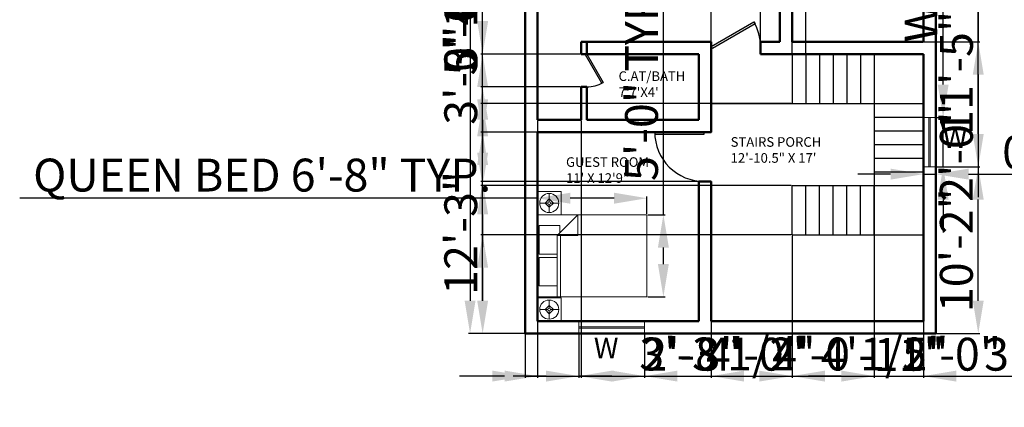
# Model space of a CAD drawing. Units: inches. Extents: x 1383 to 2465, y 1661 to 2415.
# Tile 1 of 4: x 1383 to 2102, y 1661 to 1944. Entities that reach past the tile are written whole.
import ezdxf

# ---------------------------------------------------------------- set-up
doc = ezdxf.new("R2010")
doc.units = ezdxf.units.IN
for name, color, linetype, lineweight in [('A-ANNO-DIMS', 2, 'Continuous', 18), ('A-ANNO-TEXT', 3, 'Continuous', 18), ('A-AREA-IDEN', 7, 'Continuous', 25), ('A-DOOR', 3, 'Continuous', 25), ('A-FLOR-STRS', 7, 'Continuous', 25), ('A-FURN', 8, 'Continuous', 18), ('A-GLAZ', 4, 'Continuous', 18), ('A-WALL', 7, 'Continuous', 50)]:
    doc.layers.add(name, color=color, linetype=linetype, lineweight=lineweight)
doc.styles.get("Standard").update_dxf_attribs({"font": 'arial.ttf'})
doc.dimstyles.new('ISO-25', dxfattribs={"dimtxt": 24, "dimasz": 24, "dimexe": 1.25, "dimexo": 0.625, "dimtad": 1, "dimdec": 0, "dimlunit": 3, "dimtxsty": 'Standard', "dimcen": 2.5, "dimadec": 0, "dimazin": 0, "dimtfac": 1, "dimtdec": 0, "dimtmove": 0, "dimatfit": 3, "dimfxl": 1, "dimarcsym": 0})

# ---------------------------------------------------------------- blocks, each defined once
blk = doc.blocks.new('*U7')
for p, q in [((0, 0), (0, -6)), ((40, 0), (40, -6))]:
    blk.add_line(p, q)
blk.add_lwpolyline([(0, 0), (34.64, 20), (35.52, 18.48), (0.87, -1.52)], close=True)
blk.add_arc((0, 0), 40, 0, 30)
blk = doc.blocks.new('*U6')
for p, q in [((0, 0), (0, 6)), ((40, 0), (40, 6))]:
    blk.add_line(p, q)
blk.add_lwpolyline([(0, 0), (0, -40), (1.75, -40), (1.75, 0)], close=True)
blk.add_arc((0, 0), 40, 270, 0)
blk = doc.blocks.new('*U3')
for p, q in [((0, 0), (0, -6)), ((40, 0), (40, -6))]:
    blk.add_line(p, q)
blk.add_lwpolyline([(0, 0), (34.6, 20), (35.5, 18.5), (0.9, -1.5)], close=True)
blk.add_arc((0, 0), 40, 0, 30)
blk = doc.blocks.new('Bed - Queen')
for p, q in [((0, -80.00003), (0, 0)), ((0, 0), (59.99999, 0)), ((59.99999, 0), (59.99999, -80.00003)), ((7.99999, -1.2), (28.79998, -1.2)), ((7.99999, -14.4), (7.99999, -1.2)), ((28.79998, -1.2), (28.79998, -14.4)), ((31.19999, -1.2), (51.99999, -1.2)), ((31.19999, -14.4), (31.19999, -1.2)), ((51.99999, -1.2), (51.99999, -16.4)), ((0, -14.4), (44.8, -14.4)), ((44.8, -16.8), (0, -16.8)), ((59.99999, -29.6), (44.8, -14.4)), ((44.8, -14.4), (44.8, -29.6)), ((51.99999, -16.4), (46.79936, -16.4)), ((44.8, -29.6), (59.99999, -29.6)), ((59.99999, -80.00003), (0, -80.00003))]:
    blk.add_line(p, q)
blk = doc.blocks.new('*D13')
at = {"layer": 'A-ANNO-DIMS', "color": 0, "lineweight": -2, "transparency": 16777216}
for p, q in [((1751.57, 2255.16), (1710.71, 2255.16)), ((1711.96, 2231.16), (1711.96, 1739.16)), ((1751.57, 1715.16), (1710.71, 1715.16))]:
    blk.add_line(p, q, dxfattribs=at)
at = {"layer": 'A-ANNO-DIMS', "color": 0, "transparency": 16777216}
for points in [[(1707.96, 2231.16), (1715.96, 2231.16), (1711.96, 2255.16)], [(1707.96, 1739.16), (1715.96, 1739.16), (1711.96, 1715.16)]]:
    blk.add_solid(points, dxfattribs=at)
at = {"layer": 'Defpoints', "color": 0, "transparency": 16777216}
for p in [(1752.19, 2255.16), (1711.96, 1715.16), (1752.19, 1715.16)]:
    blk.add_point(p, dxfattribs=at)
at = {"layer": 'A-ANNO-DIMS', "color": 0, "transparency": 16777216, "insert": (1699.13, 1985.16), "char_height": 24, "attachment_point": 5, "rotation": 90}
blk.add_mtext("45'", dxfattribs=at)
blk = doc.blocks.new('WIN-36IN')
for p, q in [((0, 36), (9, 36)), ((0, 0), (0, 36)), ((4, 0), (4, 36)), ((5, 36), (5, 0)), ((9, 36), (9, 0)), ((9, 0), (0, 0))]:
    blk.add_line(p, q)
blk = doc.blocks.new('Lamp - Table')
for p, q in [((-1, 0), (-7, 0)), ((0, 3), (-3, 0)), ((-3, 0), (0, -3)), ((0, 7), (0, 1)), ((3, 0), (0, 3)), ((0, -3), (3, 0)), ((1, 0), (7, 0)), ((0, -1), (0, -7))]:
    blk.add_line(p, q)
for radius in [7, 1]:
    blk.add_circle((0, 0), radius)
blk = doc.blocks.new('NIGHTSTAND-WITH-LAMP')
blk.add_lwpolyline([(0, 0), (17.23, 0), (17.23, 16.98), (0, 16.98)], close=True)
blk.add_blockref('Lamp - Table', (8.62, 8.49))
blk = doc.blocks.new('*D18')
at = {"layer": 'A-ANNO-DIMS', "color": 0, "lineweight": -2, "transparency": 16777216}
for p, q in [((2057.59, 1896.91), (2057.59, 2225.86)), ((2052.82, 1872.91), (2058.84, 1872.91)), ((2057.59, 1836.91), (2057.59, 1872.91)), ((2052.82, 1836.91), (2058.84, 1836.91)), ((2057.59, 1812.91), (2057.59, 1788.91))]:
    blk.add_line(p, q, dxfattribs=at)
at = {"layer": 'A-ANNO-DIMS', "color": 0, "transparency": 16777216}
for points in [[(2053.59, 1896.91), (2061.59, 1896.91), (2057.59, 1872.91)], [(2053.59, 1812.91), (2061.59, 1812.91), (2057.59, 1836.91)]]:
    blk.add_solid(points, dxfattribs=at)
at = {"layer": 'Defpoints', "color": 0, "transparency": 16777216}
for p in [(2052.19, 1872.91), (2057.59, 1872.91), (2052.19, 1836.91)]:
    blk.add_point(p, dxfattribs=at)
at = {"layer": 'A-ANNO-DIMS', "color": 0, "transparency": 16777216, "insert": (2044.54, 2073.39), "char_height": 24, "attachment_point": 5, "rotation": 90}
blk.add_mtext('WINDOW 3\'-0" TYP.', dxfattribs=at)
blk = doc.blocks.new('*D19')
at = {"layer": 'A-ANNO-DIMS', "color": 0, "lineweight": -2, "transparency": 16777216}
for p, q in [((2043.19, 1836.29), (2043.19, 1830.26)), ((2052.19, 1836.29), (2052.19, 1830.26)), ((2019.19, 1831.51), (1995.19, 1831.51)), ((2043.19, 1831.51), (2052.19, 1831.51)), ((2076.19, 1831.51), (2247.74, 1831.51))]:
    blk.add_line(p, q, dxfattribs=at)
at = {"layer": 'A-ANNO-DIMS', "color": 0, "transparency": 16777216}
for points in [[(2019.19, 1835.51), (2019.19, 1827.51), (2043.19, 1831.51)], [(2076.19, 1835.51), (2076.19, 1827.51), (2052.19, 1831.51)]]:
    blk.add_solid(points, dxfattribs=at)
at = {"layer": 'Defpoints', "color": 0, "transparency": 16777216}
for p in [(2043.19, 1836.91), (2052.19, 1836.91), (2052.19, 1831.51)]:
    blk.add_point(p, dxfattribs=at)
at = {"layer": 'A-ANNO-DIMS', "color": 0, "transparency": 16777216, "insert": (2173.96, 1844.39), "char_height": 24, "attachment_point": 5}
blk.add_mtext('0\'-9" TYP.', dxfattribs=at)
blk = doc.blocks.new('*D20')
at = {"layer": 'A-ANNO-DIMS', "color": 0, "lineweight": -2, "transparency": 16777216}
for p, q in [((1761.19, 1813.92), (1382.9, 1813.92)), ((1761.19, 1802.55), (1761.19, 1815.17)), ((1817.19, 1813.92), (1785.19, 1813.92)), ((1841.19, 1802.55), (1841.19, 1815.17))]:
    blk.add_line(p, q, dxfattribs=at)
at = {"layer": 'A-ANNO-DIMS', "color": 0, "transparency": 16777216}
for points in [[(1785.19, 1817.92), (1785.19, 1809.92), (1761.19, 1813.92)], [(1817.19, 1817.92), (1817.19, 1809.92), (1841.19, 1813.92)]]:
    blk.add_solid(points, dxfattribs=at)
at = {"layer": 'Defpoints', "color": 0, "transparency": 16777216}
for p in [(1761.19, 1813.92), (1761.19, 1801.92), (1841.19, 1801.92)]:
    blk.add_point(p, dxfattribs=at)
at = {"layer": 'A-ANNO-DIMS', "color": 0, "transparency": 16777216, "insert": (1560.05, 1827.7), "char_height": 24, "attachment_point": 5}
blk.add_mtext('QUEEN BED 6\'-8" TYP.', dxfattribs=at)
blk = doc.blocks.new('*D21')
at = {"layer": 'A-ANNO-DIMS', "color": 0, "lineweight": -2, "transparency": 16777216}
for p, q in [((1853.19, 1801.92), (1853.19, 1973.47)), ((1841.82, 1801.92), (1854.44, 1801.92)), ((1853.19, 1765.92), (1853.19, 1777.92)), ((1841.82, 1741.92), (1854.44, 1741.92))]:
    blk.add_line(p, q, dxfattribs=at)
at = {"layer": 'A-ANNO-DIMS', "color": 0, "transparency": 16777216}
for points in [[(1849.19, 1777.92), (1857.19, 1777.92), (1853.19, 1801.92)], [(1849.19, 1765.92), (1857.19, 1765.92), (1853.19, 1741.92)]]:
    blk.add_solid(points, dxfattribs=at)
at = {"layer": 'Defpoints', "color": 0, "transparency": 16777216}
for p in [(1841.19, 1801.92), (1853.19, 1801.92), (1841.19, 1741.92)]:
    blk.add_point(p, dxfattribs=at)
at = {"layer": 'A-ANNO-DIMS', "color": 0, "transparency": 16777216, "insert": (1840.32, 1899.7), "char_height": 24, "attachment_point": 5, "rotation": 90}
blk.add_mtext('5\'-0" TYP.', dxfattribs=at)
blk = doc.blocks.new('*D22')
at = {"layer": 'A-ANNO-DIMS', "color": 0, "lineweight": -2, "transparency": 16777216}
for p, q in [((1888.19, 1723.54), (1888.19, 1682.86)), ((1839.47, 1714.54), (1839.47, 1682.86)), ((1815.47, 1684.11), (1791.47, 1684.11)), ((1839.47, 1684.11), (1888.19, 1684.11)), ((1912.19, 1684.11), (2058.13, 1684.11))]:
    blk.add_line(p, q, dxfattribs=at)
at = {"layer": 'A-ANNO-DIMS', "color": 0, "transparency": 16777216}
for points in [[(1815.47, 1688.11), (1815.47, 1680.11), (1839.47, 1684.11)], [(1912.19, 1688.11), (1912.19, 1680.11), (1888.19, 1684.11)]]:
    blk.add_solid(points, dxfattribs=at)
at = {"layer": 'Defpoints', "color": 0, "transparency": 16777216}
for p in [(1888.19, 1724.16), (1839.47, 1715.16), (1888.19, 1684.11)]:
    blk.add_point(p, dxfattribs=at)
at = {"layer": 'A-ANNO-DIMS', "color": 0, "transparency": 16777216, "insert": (1997.16, 1697.15), "char_height": 24, "attachment_point": 5}
blk.add_mtext('4\'-0 1/2"', dxfattribs=at)
blk = doc.blocks.new('*D23')
at = {"layer": 'A-ANNO-DIMS', "color": 0, "lineweight": -2, "transparency": 16777216}
for p, q in [((1760.57, 1862.16), (1719.89, 1862.16)), ((1721.14, 1739.16), (1721.14, 1838.16)), ((1751.57, 1715.16), (1719.89, 1715.16))]:
    blk.add_line(p, q, dxfattribs=at)
at = {"layer": 'A-ANNO-DIMS', "color": 0, "transparency": 16777216}
for points in [[(1717.14, 1838.16), (1725.14, 1838.16), (1721.14, 1862.16)], [(1717.14, 1739.16), (1725.14, 1739.16), (1721.14, 1715.16)]]:
    blk.add_solid(points, dxfattribs=at)
at = {"layer": 'Defpoints', "color": 0, "transparency": 16777216}
for p in [(1721.14, 1862.16), (1761.19, 1862.16), (1752.19, 1715.16)]:
    blk.add_point(p, dxfattribs=at)
at = {"layer": 'A-ANNO-DIMS', "color": 0, "transparency": 16777216, "insert": (1708.26, 1788.66), "char_height": 24, "attachment_point": 5, "rotation": 90}
blk.add_mtext('12\'-3"', dxfattribs=at)
blk = doc.blocks.new('*D24')
at = {"layer": 'A-ANNO-DIMS', "color": 0, "lineweight": -2, "transparency": 16777216}
for p, q in [((1721.14, 1919.16), (1721.14, 2009.18)), ((1792.57, 1919.16), (1719.89, 1919.16)), ((1721.14, 1886.16), (1721.14, 1895.16)), ((1760.57, 1862.16), (1719.89, 1862.16))]:
    blk.add_line(p, q, dxfattribs=at)
at = {"layer": 'A-ANNO-DIMS', "color": 0, "transparency": 16777216}
for points in [[(1717.14, 1895.16), (1725.14, 1895.16), (1721.14, 1919.16)], [(1717.14, 1886.16), (1725.14, 1886.16), (1721.14, 1862.16)]]:
    blk.add_solid(points, dxfattribs=at)
at = {"layer": 'Defpoints', "color": 0, "transparency": 16777216}
for p in [(1721.14, 1919.16), (1793.19, 1919.16), (1761.19, 1862.16)]:
    blk.add_point(p, dxfattribs=at)
at = {"layer": 'A-ANNO-DIMS', "color": 0, "transparency": 16777216, "insert": (1708.26, 1976.17), "char_height": 24, "attachment_point": 5, "rotation": 90}
blk.add_mtext('4\'-9"', dxfattribs=at)
blk = doc.blocks.new('*D25')
at = {"layer": 'A-ANNO-DIMS', "color": 0, "lineweight": -2, "transparency": 16777216}
for p, q in [((1760.57, 2048.16), (1719.89, 2048.16)), ((1721.14, 1943.16), (1721.14, 2024.16)), ((1792.57, 1919.16), (1719.89, 1919.16))]:
    blk.add_line(p, q, dxfattribs=at)
at = {"layer": 'A-ANNO-DIMS', "color": 0, "transparency": 16777216}
for points in [[(1717.14, 2024.16), (1725.14, 2024.16), (1721.14, 2048.16)], [(1717.14, 1943.16), (1725.14, 1943.16), (1721.14, 1919.16)]]:
    blk.add_solid(points, dxfattribs=at)
at = {"layer": 'Defpoints', "color": 0, "transparency": 16777216}
for p in [(1721.14, 2048.16), (1761.19, 2048.16), (1793.19, 1919.16)]:
    blk.add_point(p, dxfattribs=at)
at = {"layer": 'A-ANNO-DIMS', "color": 0, "transparency": 16777216, "insert": (1708.26, 1983.66), "char_height": 24, "attachment_point": 5, "rotation": 90}
blk.add_mtext('10\'-9"', dxfattribs=at)
blk = doc.blocks.new('*D31')
at = {"layer": 'A-ANNO-DIMS', "color": 0, "lineweight": -2, "transparency": 16777216}
for p, q in [((2052.82, 1836.91), (2084.49, 1836.91)), ((2083.24, 1739.16), (2083.24, 1812.91)), ((2052.82, 1715.16), (2084.49, 1715.16))]:
    blk.add_line(p, q, dxfattribs=at)
at = {"layer": 'A-ANNO-DIMS', "color": 0, "transparency": 16777216}
for points in [[(2079.24, 1812.91), (2087.24, 1812.91), (2083.24, 1836.91)], [(2079.24, 1739.16), (2087.24, 1739.16), (2083.24, 1715.16)]]:
    blk.add_solid(points, dxfattribs=at)
at = {"layer": 'Defpoints', "color": 0, "transparency": 16777216}
for p in [(2052.19, 1836.91), (2083.24, 1836.91), (2052.19, 1715.16)]:
    blk.add_point(p, dxfattribs=at)
at = {"layer": 'A-ANNO-DIMS', "color": 0, "transparency": 16777216, "insert": (2070.36, 1776.04), "char_height": 24, "attachment_point": 5, "rotation": 90}
blk.add_mtext('10\'-2"', dxfattribs=at)
blk = doc.blocks.new('*D32')
at = {"layer": 'A-ANNO-DIMS', "color": 0, "lineweight": -2, "transparency": 16777216}
for p, q in [((2052.82, 1973.98), (2084.49, 1973.98)), ((2083.24, 1860.91), (2083.24, 1949.98)), ((2052.82, 1836.91), (2084.49, 1836.91))]:
    blk.add_line(p, q, dxfattribs=at)
at = {"layer": 'A-ANNO-DIMS', "color": 0, "transparency": 16777216}
for points in [[(2079.24, 1949.98), (2087.24, 1949.98), (2083.24, 1973.98)], [(2079.24, 1860.91), (2087.24, 1860.91), (2083.24, 1836.91)]]:
    blk.add_solid(points, dxfattribs=at)
at = {"layer": 'Defpoints', "color": 0, "transparency": 16777216}
for p in [(2052.19, 1973.98), (2083.24, 1973.98), (2052.19, 1836.91)]:
    blk.add_point(p, dxfattribs=at)
at = {"layer": 'A-ANNO-DIMS', "color": 0, "transparency": 16777216, "insert": (2070.36, 1905.44), "char_height": 24, "attachment_point": 5, "rotation": 90}
blk.add_mtext('11\'-5"', dxfattribs=at)
blk = doc.blocks.new('*D36')
at = {"layer": 'A-ANNO-DIMS', "color": 0, "lineweight": -2, "transparency": 16777216}
for p, q in [((1752.19, 1714.54), (1752.19, 1682.86)), ((1791.47, 1714.54), (1791.47, 1682.86)), ((1728.19, 1684.11), (1704.19, 1684.11)), ((1752.19, 1684.11), (1791.47, 1684.11)), ((1815.47, 1684.11), (1960.42, 1684.11))]:
    blk.add_line(p, q, dxfattribs=at)
at = {"layer": 'A-ANNO-DIMS', "color": 0, "transparency": 16777216}
for points in [[(1728.19, 1688.11), (1728.19, 1680.11), (1752.19, 1684.11)], [(1815.47, 1688.11), (1815.47, 1680.11), (1791.47, 1684.11)]]:
    blk.add_solid(points, dxfattribs=at)
at = {"layer": 'Defpoints', "color": 0, "transparency": 16777216}
for p in [(1752.19, 1715.16), (1791.47, 1715.16), (1791.47, 1684.11)]:
    blk.add_point(p, dxfattribs=at)
at = {"layer": 'A-ANNO-DIMS', "color": 0, "transparency": 16777216, "insert": (1899.95, 1697.15), "char_height": 24, "attachment_point": 5}
blk.add_mtext('3\'-3 1/2"', dxfattribs=at)
blk = doc.blocks.new('*D37')
at = {"layer": 'A-ANNO-DIMS', "color": 0, "lineweight": -2, "transparency": 16777216}
for p, q in [((1791.47, 1714.54), (1791.47, 1682.86)), ((1839.47, 1714.54), (1839.47, 1682.86)), ((1767.47, 1684.11), (1743.47, 1684.11)), ((1791.47, 1684.11), (1839.47, 1684.11)), ((1863.47, 1684.11), (1953.48, 1684.11))]:
    blk.add_line(p, q, dxfattribs=at)
at = {"layer": 'A-ANNO-DIMS', "color": 0, "transparency": 16777216}
for points in [[(1767.47, 1688.11), (1767.47, 1680.11), (1791.47, 1684.11)], [(1863.47, 1688.11), (1863.47, 1680.11), (1839.47, 1684.11)]]:
    blk.add_solid(points, dxfattribs=at)
at = {"layer": 'Defpoints', "color": 0, "transparency": 16777216}
for p in [(1791.47, 1715.16), (1839.47, 1715.16), (1839.47, 1684.11)]:
    blk.add_point(p, dxfattribs=at)
at = {"layer": 'A-ANNO-DIMS', "color": 0, "transparency": 16777216, "insert": (1920.48, 1696.99), "char_height": 24, "attachment_point": 5}
blk.add_mtext('4\'-0"', dxfattribs=at)
blk = doc.blocks.new('*D41')
at = {"layer": 'A-ANNO-DIMS', "color": 0, "lineweight": -2, "transparency": 16777216}
for p, q in [((1721.14, 1943.16), (1721.14, 2032.62)), ((1792.57, 1919.16), (1719.89, 1919.16)), ((1721.14, 1895.16), (1721.14, 1919.16)), ((1792.57, 1895.16), (1719.89, 1895.16)), ((1721.14, 1871.16), (1721.14, 1847.16))]:
    blk.add_line(p, q, dxfattribs=at)
at = {"layer": 'A-ANNO-DIMS', "color": 0, "transparency": 16777216}
for points in [[(1717.14, 1943.16), (1725.14, 1943.16), (1721.14, 1919.16)], [(1717.14, 1871.16), (1725.14, 1871.16), (1721.14, 1895.16)]]:
    blk.add_solid(points, dxfattribs=at)
at = {"layer": 'Defpoints', "color": 0, "transparency": 16777216}
for p in [(1721.14, 1919.16), (1793.19, 1919.16), (1793.19, 1895.16)]:
    blk.add_point(p, dxfattribs=at)
at = {"layer": 'A-ANNO-DIMS', "color": 0, "transparency": 16777216, "insert": (1708.26, 1999.89), "char_height": 24, "attachment_point": 5, "rotation": 90}
blk.add_mtext('2\'-0"', dxfattribs=at)
blk = doc.blocks.new('*D42')
at = {"layer": 'A-ANNO-DIMS', "color": 0, "lineweight": -2, "transparency": 16777216}
for p, q in [((1761.19, 1870.54), (1761.19, 1682.86)), ((1793.19, 1870.54), (1793.19, 1682.86)), ((1737.19, 1684.11), (1713.19, 1684.11)), ((1761.19, 1684.11), (1793.19, 1684.11)), ((1817.19, 1684.11), (1906.65, 1684.11))]:
    blk.add_line(p, q, dxfattribs=at)
at = {"layer": 'A-ANNO-DIMS', "color": 0, "transparency": 16777216}
for points in [[(1737.19, 1688.11), (1737.19, 1680.11), (1761.19, 1684.11)], [(1817.19, 1688.11), (1817.19, 1680.11), (1793.19, 1684.11)]]:
    blk.add_solid(points, dxfattribs=at)
at = {"layer": 'Defpoints', "color": 0, "transparency": 16777216}
for p in [(1761.19, 1871.16), (1793.19, 1871.16), (1793.19, 1684.11)]:
    blk.add_point(p, dxfattribs=at)
at = {"layer": 'A-ANNO-DIMS', "color": 0, "transparency": 16777216, "insert": (1873.92, 1696.99), "char_height": 24, "attachment_point": 5}
blk.add_mtext('2\'-8"', dxfattribs=at)
blk = doc.blocks.new('*D43')
at = {"layer": 'A-ANNO-DIMS', "color": 0, "lineweight": -2, "transparency": 16777216}
for p, q in [((1923.19, 2286.21), (1899.19, 2286.21)), ((1947.19, 1919.79), (1947.19, 2287.46)), ((1947.19, 2286.21), (1957.19, 2286.21)), ((1957.19, 1919.79), (1957.19, 2287.46)), ((1981.19, 2286.21), (2088.89, 2286.21))]:
    blk.add_line(p, q, dxfattribs=at)
at = {"layer": 'A-ANNO-DIMS', "color": 0, "transparency": 16777216}
for points in [[(1923.19, 2290.21), (1923.19, 2282.21), (1947.19, 2286.21)], [(1981.19, 2290.21), (1981.19, 2282.21), (1957.19, 2286.21)]]:
    blk.add_solid(points, dxfattribs=at)
at = {"layer": 'Defpoints', "color": 0, "transparency": 16777216}
for p in [(1957.19, 2286.21), (1947.19, 1919.16), (1957.19, 1919.16)]:
    blk.add_point(p, dxfattribs=at)
at = {"layer": 'A-ANNO-DIMS', "color": 0, "transparency": 16777216, "insert": (2047.04, 2299.09), "char_height": 24, "attachment_point": 5}
blk.add_mtext('0\'-10"', dxfattribs=at)
blk = doc.blocks.new('*D44')
at = {"layer": 'A-ANNO-DIMS', "color": 0, "lineweight": -2, "transparency": 16777216}
for p, q in [((1721.14, 1847.16), (1721.14, 1936.19)), ((1946.57, 1823.16), (1719.89, 1823.16)), ((1721.14, 1787.16), (1721.14, 1823.16)), ((1946.57, 1787.16), (1719.89, 1787.16)), ((1721.14, 1763.16), (1721.14, 1739.16))]:
    blk.add_line(p, q, dxfattribs=at)
at = {"layer": 'A-ANNO-DIMS', "color": 0, "transparency": 16777216}
for points in [[(1717.14, 1847.16), (1725.14, 1847.16), (1721.14, 1823.16)], [(1717.14, 1763.16), (1725.14, 1763.16), (1721.14, 1787.16)]]:
    blk.add_solid(points, dxfattribs=at)
at = {"layer": 'Defpoints', "color": 0, "transparency": 16777216}
for p in [(1721.14, 1823.16), (1947.19, 1823.16), (1947.19, 1787.16)]:
    blk.add_point(p, dxfattribs=at)
at = {"layer": 'A-ANNO-DIMS', "color": 0, "transparency": 16777216, "insert": (1708.26, 1903.68), "char_height": 24, "attachment_point": 5, "rotation": 90}
blk.add_mtext('3\'-0"', dxfattribs=at)
blk = doc.blocks.new('*D45')
at = {"layer": 'A-ANNO-DIMS', "color": 0, "lineweight": -2, "transparency": 16777216}
for p, q in [((1947.19, 1786.54), (1947.19, 1682.86)), ((2007.19, 1786.54), (2007.19, 1682.86)), ((1971.19, 1684.11), (1983.19, 1684.11)), ((2007.19, 1684.11), (2096.24, 1684.11))]:
    blk.add_line(p, q, dxfattribs=at)
at = {"layer": 'A-ANNO-DIMS', "color": 0, "transparency": 16777216}
for points in [[(1971.19, 1688.11), (1971.19, 1680.11), (1947.19, 1684.11)], [(1983.19, 1688.11), (1983.19, 1680.11), (2007.19, 1684.11)]]:
    blk.add_solid(points, dxfattribs=at)
at = {"layer": 'Defpoints', "color": 0, "transparency": 16777216}
for p in [(1947.19, 1787.16), (2007.19, 1787.16), (2007.19, 1684.11)]:
    blk.add_point(p, dxfattribs=at)
at = {"layer": 'A-ANNO-DIMS', "color": 0, "transparency": 16777216, "insert": (2063.72, 1696.99), "char_height": 24, "attachment_point": 5}
blk.add_mtext('5\'-0"', dxfattribs=at)
blk = doc.blocks.new('*D46')
at = {"layer": 'A-ANNO-DIMS', "color": 0, "lineweight": -2, "transparency": 16777216}
for p, q in [((2007.19, 1786.54), (2007.19, 1682.86)), ((2043.19, 1786.54), (2043.19, 1682.86)), ((1983.19, 1684.11), (1959.19, 1684.11)), ((2007.19, 1684.11), (2043.19, 1684.11)), ((2067.19, 1684.11), (2156.23, 1684.11))]:
    blk.add_line(p, q, dxfattribs=at)
at = {"layer": 'A-ANNO-DIMS', "color": 0, "transparency": 16777216}
for points in [[(1983.19, 1688.11), (1983.19, 1680.11), (2007.19, 1684.11)], [(2067.19, 1688.11), (2067.19, 1680.11), (2043.19, 1684.11)]]:
    blk.add_solid(points, dxfattribs=at)
at = {"layer": 'Defpoints', "color": 0, "transparency": 16777216}
for p in [(2007.19, 1787.16), (2043.19, 1787.16), (2043.19, 1684.11)]:
    blk.add_point(p, dxfattribs=at)
at = {"layer": 'A-ANNO-DIMS', "color": 0, "transparency": 16777216, "insert": (2123.71, 1697), "char_height": 24, "attachment_point": 5}
blk.add_mtext('3\'-0"', dxfattribs=at)
blk = doc.blocks.new('*D47')
at = {"layer": 'A-ANNO-DIMS', "color": 0, "lineweight": -2, "transparency": 16777216}
for p, q in [((1721.14, 1883.16), (1721.14, 1972.21)), ((1946.57, 1883.16), (1719.89, 1883.16)), ((1721.14, 1847.16), (1721.14, 1859.16)), ((1946.57, 1823.16), (1719.89, 1823.16))]:
    blk.add_line(p, q, dxfattribs=at)
at = {"layer": 'A-ANNO-DIMS', "color": 0, "transparency": 16777216}
for points in [[(1717.14, 1859.16), (1725.14, 1859.16), (1721.14, 1883.16)], [(1717.14, 1847.16), (1725.14, 1847.16), (1721.14, 1823.16)]]:
    blk.add_solid(points, dxfattribs=at)
at = {"layer": 'Defpoints', "color": 0, "transparency": 16777216}
for p in [(1721.14, 1883.16), (1947.19, 1883.16), (1947.19, 1823.16)]:
    blk.add_point(p, dxfattribs=at)
at = {"layer": 'A-ANNO-DIMS', "color": 0, "transparency": 16777216, "insert": (1708.26, 1939.69), "char_height": 24, "attachment_point": 5, "rotation": 90}
blk.add_mtext('5\'-0"', dxfattribs=at)
blk = doc.blocks.new('*D50')
at = {"layer": 'A-ANNO-DIMS', "color": 0, "lineweight": -2, "transparency": 16777216}
for p, q in [((1864.19, 2286.21), (1840.19, 2286.21)), ((1888.19, 1919.79), (1888.19, 2287.46)), ((1888.19, 2286.21), (1924.19, 2286.21)), ((1924.19, 1919.79), (1924.19, 2287.46)), ((1948.19, 2286.21), (2037.23, 2286.21))]:
    blk.add_line(p, q, dxfattribs=at)
at = {"layer": 'A-ANNO-DIMS', "color": 0, "transparency": 16777216}
for points in [[(1864.19, 2290.21), (1864.19, 2282.21), (1888.19, 2286.21)], [(1948.19, 2290.21), (1948.19, 2282.21), (1924.19, 2286.21)]]:
    blk.add_solid(points, dxfattribs=at)
at = {"layer": 'Defpoints', "color": 0, "transparency": 16777216}
for p in [(1924.19, 2286.21), (1888.19, 1919.16), (1924.19, 1919.16)]:
    blk.add_point(p, dxfattribs=at)
at = {"layer": 'A-ANNO-DIMS', "color": 0, "transparency": 16777216, "insert": (2004.71, 2299.1), "char_height": 24, "attachment_point": 5}
blk.add_mtext('3\'-0"', dxfattribs=at)
blk = doc.blocks.new('*D51')
at = {"layer": 'A-ANNO-DIMS', "color": 0, "lineweight": -2, "transparency": 16777216}
for p, q in [((1888.19, 1825.54), (1888.19, 1682.86)), ((1947.19, 1786.54), (1947.19, 1682.86)), ((1912.19, 1684.11), (1923.19, 1684.11)), ((1947.19, 1684.11), (2055.85, 1684.11))]:
    blk.add_line(p, q, dxfattribs=at)
at = {"layer": 'A-ANNO-DIMS', "color": 0, "transparency": 16777216}
for points in [[(1912.19, 1688.11), (1912.19, 1680.11), (1888.19, 1684.11)], [(1923.19, 1688.11), (1923.19, 1680.11), (1947.19, 1684.11)]]:
    blk.add_solid(points, dxfattribs=at)
at = {"layer": 'Defpoints', "color": 0, "transparency": 16777216}
for p in [(1888.19, 1826.16), (1947.19, 1787.16), (1947.19, 1684.11)]:
    blk.add_point(p, dxfattribs=at)
at = {"layer": 'A-ANNO-DIMS', "color": 0, "transparency": 16777216, "insert": (2013.52, 1696.79), "char_height": 24, "attachment_point": 5}
blk.add_mtext('4\'-11"', dxfattribs=at)
blk = doc.blocks.new('*D52')
at = {"layer": 'A-ANNO-DIMS', "color": 0, "lineweight": -2, "transparency": 16777216}
for p, q in [((2083.24, 1976.16), (2083.24, 2000.16)), ((2019.82, 1952.16), (2084.49, 1952.16)), ((2083.24, 1952.16), (2083.24, 1928.16)), ((2043.82, 1928.16), (2084.49, 1928.16)), ((2083.24, 1904.16), (2083.24, 1814.7))]:
    blk.add_line(p, q, dxfattribs=at)
at = {"layer": 'A-ANNO-DIMS', "color": 0, "transparency": 16777216}
for points in [[(2079.24, 1976.16), (2087.24, 1976.16), (2083.24, 1952.16)], [(2079.24, 1904.16), (2087.24, 1904.16), (2083.24, 1928.16)]]:
    blk.add_solid(points, dxfattribs=at)
at = {"layer": 'Defpoints', "color": 0, "transparency": 16777216}
for p in [(2019.19, 1952.16), (2043.19, 1928.16), (2083.24, 1928.16)]:
    blk.add_point(p, dxfattribs=at)
at = {"layer": 'A-ANNO-DIMS', "color": 0, "transparency": 16777216, "insert": (2070.36, 1847.43), "char_height": 24, "attachment_point": 5, "rotation": 90}
blk.add_mtext('2\'-0"', dxfattribs=at)
blk = doc.blocks.new('*D53')
at = {"layer": 'A-ANNO-DIMS', "color": 0, "lineweight": -2, "transparency": 16777216}
for p, q in [((1721.14, 1886.16), (1721.14, 1975.19)), ((1887.57, 1862.16), (1719.89, 1862.16)), ((1721.14, 1826.16), (1721.14, 1862.16)), ((1887.57, 1826.16), (1719.89, 1826.16)), ((1721.14, 1802.16), (1721.14, 1778.16))]:
    blk.add_line(p, q, dxfattribs=at)
at = {"layer": 'A-ANNO-DIMS', "color": 0, "transparency": 16777216}
for points in [[(1717.14, 1886.16), (1725.14, 1886.16), (1721.14, 1862.16)], [(1717.14, 1802.16), (1725.14, 1802.16), (1721.14, 1826.16)]]:
    blk.add_solid(points, dxfattribs=at)
at = {"layer": 'Defpoints', "color": 0, "transparency": 16777216}
for p in [(1721.14, 1862.16), (1888.19, 1862.16), (1888.19, 1826.16)]:
    blk.add_point(p, dxfattribs=at)
at = {"layer": 'A-ANNO-DIMS', "color": 0, "transparency": 16777216, "insert": (1708.26, 1942.68), "char_height": 24, "attachment_point": 5, "rotation": 90}
blk.add_mtext('3\'-0"', dxfattribs=at)

msp = doc.modelspace()

# ---------------------------------------------------------------- linework, layer by layer
at = {"layer": 'A-FLOR-STRS'}
for p, q in [((1947.19, 1919.16), (1947.19, 1883.16)), ((1957.19, 1919.16), (1957.19, 1883.16)), ((1967.19, 1919.16), (1967.19, 1883.16)), ((1977.19, 1919.16), (1977.19, 1883.16)), ((1987.19, 1919.16), (1987.19, 1883.16)), ((1997.19, 1919.16), (1997.19, 1883.16)), ((2007.19, 1919.16), (2007.19, 1787.16)), ((1888.19, 1883.16), (2043.19, 1883.16)), ((2007.19, 1883.16), (2043.19, 1883.16)), ((2007.19, 1873.16), (2043.19, 1873.16)), ((2007.19, 1863.16), (2043.19, 1863.16)), ((2007.19, 1853.16), (2043.19, 1853.16)), ((2007.19, 1843.16), (2043.19, 1843.16)), ((2007.19, 1833.16), (2043.19, 1833.16)), ((1947.19, 1823.16), (2043.19, 1823.16)), ((1947.19, 1787.16), (1947.19, 1823.16)), ((1957.19, 1787.16), (1957.19, 1823.16)), ((1967.19, 1787.16), (1967.19, 1823.16)), ((1977.19, 1787.16), (1977.19, 1823.16)), ((1987.19, 1787.16), (1987.19, 1823.16)), ((1997.19, 1787.16), (1997.19, 1823.16)), ((2007.19, 1787.16), (2007.19, 1823.16)), ((1947.19, 1787.16), (2043.19, 1787.16))]:
    msp.add_line(p, q, dxfattribs=at)
at = {"layer": 'A-GLAZ'}
for p, q in [((1791.47, 1715.16), (1791.47, 1724.16)), ((1791.47, 1724.16), (1839.47, 1724.16)), ((1791.47, 1720.16), (1839.47, 1720.16)), ((1839.47, 1724.16), (1839.47, 1715.16)), ((1839.47, 1719.16), (1791.47, 1719.16)), ((1839.47, 1715.16), (1791.47, 1715.16))]:
    msp.add_line(p, q, dxfattribs=at)
at = {"layer": 'A-WALL'}
for p, q in [((1761.19, 1871.16), (1761.19, 2048.16)), ((2043.19, 2048.16), (2043.19, 1928.16)), ((1938.19, 2009.16), (1938.19, 1928.16)), ((1947.19, 2009.16), (1947.19, 1928.16)), ((1793.19, 1928.16), (1888.19, 1928.16)), ((1793.19, 1919.16), (1793.19, 1928.16)), ((1797.19, 1919.16), (1797.19, 1928.16)), ((1888.19, 1919.16), (1888.19, 1928.16)), ((1888.19, 1862.16), (1888.19, 1928.16)), ((1924.19, 1919.16), (1924.19, 1928.16)), ((1924.19, 1928.16), (1938.19, 1928.16)), ((1947.19, 1928.16), (2043.19, 1928.16)), ((1793.19, 1919.16), (1879.19, 1919.16)), ((1879.19, 1871.16), (1879.19, 1919.16)), ((1924.19, 1919.16), (2043.19, 1919.16)), ((1924.19, 1919.16), (2043.19, 1919.16)), ((2043.19, 1919.16), (2043.19, 1724.16)), ((2043.19, 1919.16), (2043.19, 1724.16)), ((1793.19, 1871.16), (1793.19, 1895.16)), ((1793.19, 1895.16), (1797.19, 1895.16)), ((1797.19, 1871.16), (1797.19, 1895.16)), ((1761.19, 1871.16), (1793.19, 1871.16)), ((1797.19, 1871.16), (1879.19, 1871.16)), ((1761.19, 1724.16), (1761.19, 1862.16)), ((1761.19, 1862.16), (1888.19, 1862.16)), ((2043.19, 1862.16), (2043.19, 1724.16)), ((1879.19, 1724.16), (1879.19, 1826.16)), ((1879.19, 1826.16), (1888.19, 1826.16)), ((1888.19, 1724.16), (1888.19, 1826.16)), ((1879.19, 1724.16), (1761.19, 1724.16)), ((2043.19, 1724.16), (1888.19, 1724.16))]:
    msp.add_line(p, q, dxfattribs=at)
msp.add_lwpolyline([(1752.19, 2255.16), (2052.19, 2255.16), (2052.19, 1715.16), (1752.19, 1715.16)], close=True, dxfattribs=at)

# ---------------------------------------------------------------- block references
at = {"layer": 'A-DOOR', "xscale": 0.8999999999999948, "yscale": 0.8999999999999948, "zscale": 0.8999999999999948}
msp.add_blockref('*U7', (1888.19, 1924.56), dxfattribs=at)
at = {"layer": 'A-DOOR', "rotation": 270}
for name, p, xscale, yscale, zscale in [('*U3', (1797.19, 1919.16), 0.6, 0.6, 0.6), ('*U6', (1882.88, 1862.16), 0.8999999999999948, 0.8999999999999948, 0.8999999999999948)]:
    msp.add_blockref(name, p, dxfattribs=dict(at, xscale=xscale, yscale=yscale, zscale=zscale))
at = {"layer": 'A-FURN'}
for p in [(1761.19, 1801.92), (1761.19, 1724.16)]:
    msp.add_blockref('NIGHTSTAND-WITH-LAMP', p, dxfattribs=at)
at = {"layer": 'A-FURN', "rotation": 90}
msp.add_blockref('Bed - Queen', (1761.19, 1741.92), dxfattribs=at)
at = {"layer": 'A-GLAZ'}
msp.add_blockref('WIN-36IN', (2043.19, 1836.91), dxfattribs=at)

# ---------------------------------------------------------------- texts
at = {"layer": 'A-ANNO-TEXT', "char_height": 15, "attachment_point": 1}
for insert in [(2057.31, 1865.52), (1802.4, 1712.14)]:
    msp.add_mtext_dynamic_manual_height_columns('{\\fArial|b1|i0|c0|p34;W}', width=53.5912, gutter_width=12.5, heights=[38.86], dxfattribs=dict(at, insert=insert))
at = {"layer": 'A-AREA-IDEN', "char_height": 7, "attachment_point": 1}
for s, width, heights, insert in [("{\\fArial|b1|i0|c0|p34;C.AT/BATH\\P7'7'X4'}", 53.5912, [38.86], (1820.44, 1906.51)), ('{\\fArial|b1|i0|c0|p34;STAIRS PORCH\\P12\'-10.5" X 17\'}', 100.6887, [47.04], (1902.35, 1858.48)), ('{\\fArial|b1|i0|c0|p34;GUEST ROOM\\P11\' X 12\'9"}', 96.1109, [67.38], (1782.07, 1843.81))]:
    msp.add_mtext_dynamic_manual_height_columns(s, width=width, gutter_width=12.5, heights=heights, dxfattribs=dict(at, insert=insert))

# ---------------------------------------------------------------- dimensions: what is measured, and where the dimension line sits
at = {"layer": 'A-ANNO-DIMS'}
for base, p1, p2, picture, middle in [((1924.19, 2286.21), (1888.19, 1919.16), (1924.19, 1919.16), '*D50', (2004.71, 2299.1)), ((1957.19, 2286.21), (1947.19, 1919.16), (1957.19, 1919.16), '*D43', (2047.04, 2299.09)), ((1793.19, 1684.11), (1761.19, 1871.16), (1793.19, 1871.16), '*D42', (1873.92, 1696.99)), ((1947.19, 1684.11), (1888.19, 1826.16), (1947.19, 1787.16), '*D51', (2013.52, 1696.79)), ((2007.19, 1684.11), (1947.19, 1787.16), (2007.19, 1787.16), '*D45', (2063.72, 1696.99)), ((2043.19, 1684.11), (2007.19, 1787.16), (2043.19, 1787.16), '*D46', (2123.71, 1697)), ((1791.47, 1684.11), (1752.19, 1715.16), (1791.47, 1715.16), '*D36', (1899.95, 1697.15)), ((1888.19, 1684.11), (1839.47, 1715.16), (1888.19, 1724.16), '*D22', (1997.16, 1697.15)), ((1839.47, 1684.11), (1791.47, 1715.16), (1839.47, 1715.16), '*D37', (1920.48, 1696.99))]:
    dim = msp.add_linear_dim(base=base, p1=p1, p2=p2, dimstyle='ISO-25', override={"dimdec": 1, "dimlfac": 1, "dimrnd": 0, "dimzin": 1, "dimdsep": 46, "dimlunit": 4, "dimfrac": 2}, dxfattribs=at)
    dim.commit()
    dim.dimension.update_dxf_attribs({"geometry": picture, "text_midpoint": middle})
for base, p1, p2, override, picture, middle in [((1711.96, 1715.16), (1752.19, 2255.16), (1752.19, 1715.16), {"dimclrd": 0, "dimclre": 0, "dimclrt": 0}, '*D13', (1699.13, 1985.16)), ((1721.14, 2048.16), (1793.19, 1919.16), (1761.19, 2048.16), {"dimdec": 1, "dimlfac": 1, "dimrnd": 0, "dimzin": 1, "dimdsep": 46, "dimlunit": 4, "dimfrac": 2}, '*D25', (1708.26, 1983.66)), ((1721.14, 1919.16), (1793.19, 1895.16), (1793.19, 1919.16), {"dimdec": 1, "dimlfac": 1, "dimrnd": 0, "dimzin": 1, "dimdsep": 46, "dimlunit": 4, "dimfrac": 2}, '*D41', (1708.26, 1999.89)), ((1721.14, 1919.16), (1761.19, 1862.16), (1793.19, 1919.16), {"dimdec": 1, "dimlfac": 1, "dimrnd": 0, "dimzin": 1, "dimdsep": 46, "dimlunit": 4, "dimfrac": 2}, '*D24', (1708.26, 1976.17)), ((2083.24, 1928.16), (2019.19, 1952.16), (2043.19, 1928.16), {"dimdec": 1, "dimlfac": 1, "dimrnd": 0, "dimzin": 1, "dimdsep": 46, "dimlunit": 4, "dimfrac": 2}, '*D52', (2070.36, 1847.43)), ((1721.14, 1862.16), (1888.19, 1826.16), (1888.19, 1862.16), {"dimdec": 1, "dimlfac": 1, "dimrnd": 0, "dimzin": 1, "dimdsep": 46, "dimlunit": 4, "dimfrac": 2}, '*D53', (1708.26, 1942.68)), ((1721.14, 1883.16), (1947.19, 1823.16), (1947.19, 1883.16), {"dimdec": 1, "dimlfac": 1, "dimrnd": 0, "dimzin": 1, "dimdsep": 46, "dimlunit": 4, "dimfrac": 2}, '*D47', (1708.26, 1939.69)), ((2083.24, 1973.98), (2052.19, 1836.91), (2052.19, 1973.98), {"dimdec": 1, "dimlfac": 1, "dimrnd": 0, "dimzin": 1, "dimdsep": 46, "dimlunit": 4, "dimfrac": 2}, '*D32', (2070.36, 1905.44)), ((1721.14, 1823.16), (1947.19, 1787.16), (1947.19, 1823.16), {"dimdec": 1, "dimlfac": 1, "dimrnd": 0, "dimzin": 1, "dimdsep": 46, "dimlunit": 4, "dimfrac": 2}, '*D44', (1708.26, 1903.68)), ((1721.14, 1862.16), (1752.19, 1715.16), (1761.19, 1862.16), {"dimdec": 1, "dimlfac": 1, "dimrnd": 0, "dimzin": 1, "dimdsep": 46, "dimlunit": 4, "dimfrac": 2}, '*D23', (1708.26, 1788.66)), ((2083.2437, 1836.9143), (2052.1937, 1715.1622), (2052.1937, 1836.9143), {"dimdec": 1, "dimlfac": 1, "dimrnd": 0, "dimzin": 1, "dimdsep": 46, "dimlunit": 4, "dimfrac": 2}, '*D31', (2070.365, 1776.0383))]:
    dim = msp.add_linear_dim(base=base, p1=p1, p2=p2, angle=90, dimstyle='ISO-25', override=override, dxfattribs=at)
    dim.commit()
    dim.dimension.update_dxf_attribs({"geometry": picture, "text_midpoint": middle})
for base, p1, p2, angle, text, picture, middle in [((2057.59, 1872.91), (2052.19, 1836.91), (2052.19, 1872.91), 90, 'WINDOW <> TYP.', '*D18', (2044.54, 2073.39)), ((1853.19, 1801.92), (1841.19, 1741.92), (1841.19, 1801.92), 90, '<> TYP.', '*D21', (1840.32, 1899.7)), ((1761.19, 1813.92), (1841.19, 1801.92), (1761.19, 1801.92), 180, 'QUEEN BED <> TYP.', '*D20', (1560.05, 1827.7))]:
    dim = msp.add_linear_dim(base=base, p1=p1, p2=p2, angle=angle, text=text, dimstyle='ISO-25', override={"dimdec": 1, "dimlfac": 1, "dimrnd": 0, "dimzin": 1, "dimdsep": 46, "dimlunit": 4, "dimfrac": 2}, dxfattribs=at)
    dim.commit()
    dim.dimension.update_dxf_attribs({"geometry": picture, "text_midpoint": middle})
dim = msp.add_linear_dim(base=(2052.19, 1831.51), p1=(2043.19, 1836.91), p2=(2052.19, 1836.91), text='<> TYP.', dimstyle='ISO-25', override={"dimdec": 1, "dimlfac": 1, "dimrnd": 0, "dimzin": 1, "dimdsep": 46, "dimlunit": 4, "dimfrac": 2}, dxfattribs=at)
dim.commit()
dim.dimension.update_dxf_attribs({"geometry": '*D19', "text_midpoint": (2173.96, 1844.39)})

doc.saveas('drawing.dxf')
